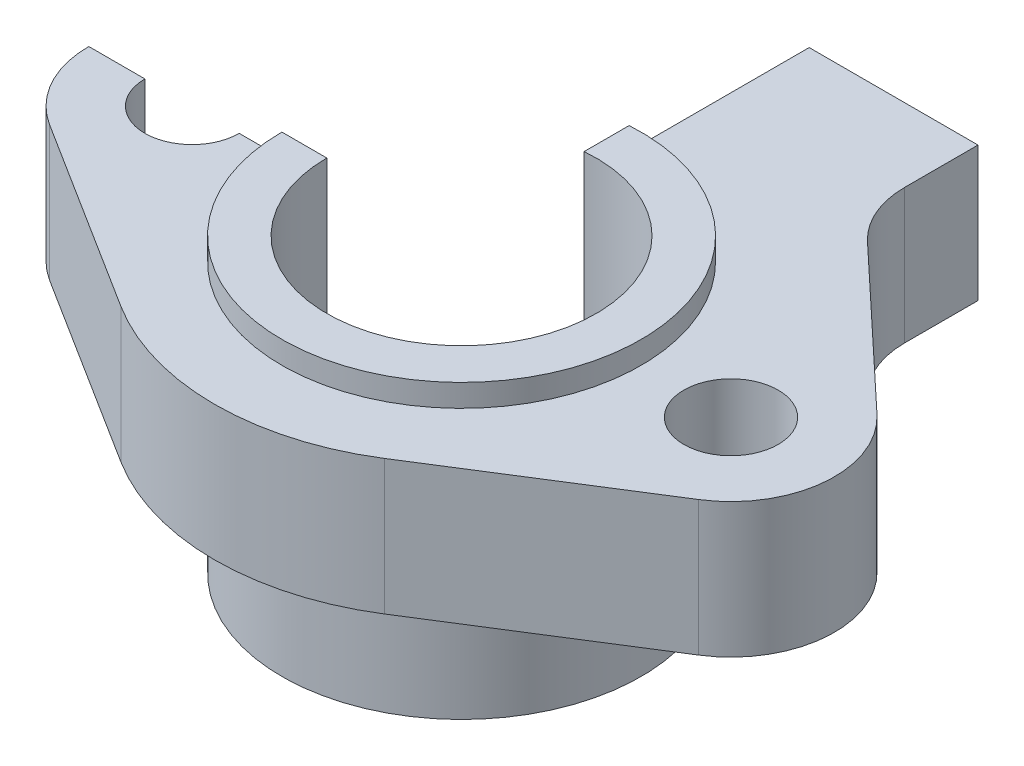
ISO-10303-21;
HEADER;
FILE_DESCRIPTION(('STEP AP214'),'2;1');
FILE_NAME('part.step','',(''),(''),'','','');
FILE_SCHEMA(('AUTOMOTIVE_DESIGN { 1 0 10303 214 1 1 1 1 }'));
ENDSEC;
DATA;
#1=APPLICATION_CONTEXT('core data for automotive mechanical design processes');
#2=APPLICATION_PROTOCOL_DEFINITION('international standard','automotive_design',2000,#1);
#3=PRODUCT_CONTEXT('',#1,'mechanical');
#4=PRODUCT('Part','Part','',(#3));
#5=PRODUCT_RELATED_PRODUCT_CATEGORY('part','',(#4));
#6=PRODUCT_DEFINITION_FORMATION('','',#4);
#7=PRODUCT_DEFINITION_CONTEXT('part definition',#1,'design');
#8=PRODUCT_DEFINITION('design','',#6,#7);
#9=PRODUCT_DEFINITION_SHAPE('','',#8);
#10=(LENGTH_UNIT() NAMED_UNIT(*) SI_UNIT(.MILLI.,.METRE.));
#11=(NAMED_UNIT(*) PLANE_ANGLE_UNIT() SI_UNIT($,.RADIAN.));
#12=(NAMED_UNIT(*) SI_UNIT($,.STERADIAN.) SOLID_ANGLE_UNIT());
#13=UNCERTAINTY_MEASURE_WITH_UNIT(LENGTH_MEASURE(1.E-05),#10,'distance_accuracy_value','');
#14=(GEOMETRIC_REPRESENTATION_CONTEXT(3) GLOBAL_UNCERTAINTY_ASSIGNED_CONTEXT((#13)) GLOBAL_UNIT_ASSIGNED_CONTEXT((#10,
#11,#12)) REPRESENTATION_CONTEXT('',''));
#15=CARTESIAN_POINT('',(0.,0.,0.));
#16=DIRECTION('',(0.,0.,1.));
#17=DIRECTION('',(1.,0.,0.));
#18=AXIS2_PLACEMENT_3D('',#15,#16,#17);
#19=CARTESIAN_POINT('',(0.,-135.,0.));
#20=DIRECTION('',(0.,0.,1.));
#21=DIRECTION('',(1.,0.,0.));
#22=AXIS2_PLACEMENT_3D('',#19,#20,#21);
#23=PLANE('',#22);
#24=DIRECTION('',(0.,1.,0.));
#25=VECTOR('',#24,1.);
#26=CARTESIAN_POINT('',(-49.5,-507.,0.));
#27=LINE('',#26,#25);
#28=CARTESIAN_POINT('',(-49.5,30.,0.));
#29=VERTEX_POINT('',#28);
#30=CARTESIAN_POINT('',(-49.5,0.,0.));
#31=VERTEX_POINT('',#30);
#32=EDGE_CURVE('E11',#29,#31,#27,.F.);
#33=ORIENTED_EDGE('',*,*,#32,.F.);
#34=DIRECTION('',(1.,0.,0.));
#35=VECTOR('',#34,1.);
#36=CARTESIAN_POINT('',(0.,30.,0.));
#37=LINE('',#36,#35);
#38=CARTESIAN_POINT('',(-40.,30.,0.));
#39=VERTEX_POINT('',#38);
#40=EDGE_CURVE('E63',#29,#39,#37,.T.);
#41=ORIENTED_EDGE('',*,*,#40,.T.);
#42=DIRECTION('',(0.,-1.,0.));
#43=VECTOR('',#42,1.);
#44=CARTESIAN_POINT('',(-40.,35.,0.));
#45=LINE('',#44,#43);
#46=CARTESIAN_POINT('',(-40.,35.,0.));
#47=VERTEX_POINT('',#46);
#48=EDGE_CURVE('E294',#47,#39,#45,.T.);
#49=ORIENTED_EDGE('',*,*,#48,.F.);
#50=DIRECTION('',(1.,0.,0.));
#51=VECTOR('',#50,1.);
#52=CARTESIAN_POINT('',(0.,35.,0.));
#53=LINE('',#52,#51);
#54=CARTESIAN_POINT('',(-30.,35.,0.));
#55=VERTEX_POINT('',#54);
#56=EDGE_CURVE('E302',#47,#55,#53,.T.);
#57=ORIENTED_EDGE('',*,*,#56,.T.);
#58=DIRECTION('',(0.,-1.,0.));
#59=VECTOR('',#58,1.);
#60=CARTESIAN_POINT('',(-30.,30.,0.));
#61=LINE('',#60,#59);
#62=CARTESIAN_POINT('',(-30.,-30.,0.));
#63=VERTEX_POINT('',#62);
#64=EDGE_CURVE('E308',#55,#63,#61,.T.);
#65=ORIENTED_EDGE('',*,*,#64,.T.);
#66=DIRECTION('',(1.,0.,0.));
#67=VECTOR('',#66,1.);
#68=CARTESIAN_POINT('',(0.,-30.,0.));
#69=LINE('',#68,#67);
#70=CARTESIAN_POINT('',(-40.,-30.,0.));
#71=VERTEX_POINT('',#70);
#72=EDGE_CURVE('E315',#71,#63,#69,.T.);
#73=ORIENTED_EDGE('',*,*,#72,.F.);
#74=DIRECTION('',(0.,-1.,0.));
#75=VECTOR('',#74,1.);
#76=CARTESIAN_POINT('',(-40.,30.,0.));
#77=LINE('',#76,#75);
#78=CARTESIAN_POINT('',(-40.,0.,0.));
#79=VERTEX_POINT('',#78);
#80=EDGE_CURVE('E190',#79,#71,#77,.T.);
#81=ORIENTED_EDGE('',*,*,#80,.F.);
#82=DIRECTION('',(1.,0.,0.));
#83=VECTOR('',#82,1.);
#84=CARTESIAN_POINT('',(0.,0.,0.));
#85=LINE('',#84,#83);
#86=EDGE_CURVE('E182',#31,#79,#85,.T.);
#87=ORIENTED_EDGE('',*,*,#86,.F.);
#88=EDGE_LOOP('',(#33,#41,#49,#57,#65,#73,#81,#87));
#89=FACE_BOUND('',#88,.T.);
#90=ADVANCED_FACE('F43',(#89),#23,.F.);
#91=DIRECTION('',(0.,1.,0.));
#92=VECTOR('',#91,1.);
#93=CARTESIAN_POINT('',(-70.5,-507.,0.));
#94=LINE('',#93,#92);
#95=CARTESIAN_POINT('',(-70.5,0.,0.));
#96=VERTEX_POINT('',#95);
#97=CARTESIAN_POINT('',(-70.5,30.,0.));
#98=VERTEX_POINT('',#97);
#99=EDGE_CURVE('E51',#96,#98,#94,.T.);
#100=ORIENTED_EDGE('',*,*,#99,.F.);
#101=CARTESIAN_POINT('',(-83.,0.,0.));
#102=VERTEX_POINT('',#101);
#103=EDGE_CURVE('E184',#102,#96,#85,.T.);
#104=ORIENTED_EDGE('',*,*,#103,.F.);
#105=DIRECTION('',(0.,1.,0.));
#106=VECTOR('',#105,1.);
#107=CARTESIAN_POINT('',(-83.,0.,0.));
#108=LINE('',#107,#106);
#109=CARTESIAN_POINT('',(-83.,30.,0.));
#110=VERTEX_POINT('',#109);
#111=EDGE_CURVE('E185',#102,#110,#108,.T.);
#112=ORIENTED_EDGE('',*,*,#111,.T.);
#113=EDGE_CURVE('E174',#110,#98,#37,.T.);
#114=ORIENTED_EDGE('',*,*,#113,.T.);
#115=EDGE_LOOP('',(#100,#104,#112,#114));
#116=FACE_BOUND('',#115,.T.);
#117=ADVANCED_FACE('F179',(#116),#23,.F.);
#118=CARTESIAN_POINT('',(0.,30.,0.));
#119=DIRECTION('',(0.,1.,0.));
#120=DIRECTION('',(0.,0.,1.));
#121=AXIS2_PLACEMENT_3D('',#118,#119,#120);
#122=PLANE('',#121);
#123=CARTESIAN_POINT('',(60.,30.,0.));
#124=DIRECTION('',(0.,1.,0.));
#125=DIRECTION('',(0.,0.,1.));
#126=AXIS2_PLACEMENT_3D('',#123,#124,#125);
#127=CIRCLE('',#126,10.5);
#128=CARTESIAN_POINT('',(60.,30.,10.5));
#129=VERTEX_POINT('',#128);
#130=EDGE_CURVE('E297',#129,#129,#127,.F.);
#131=ORIENTED_EDGE('',*,*,#130,.T.);
#132=EDGE_LOOP('',(#131));
#133=FACE_BOUND('',#132,.T.);
#134=ORIENTED_EDGE('',*,*,#40,.F.);
#135=CARTESIAN_POINT('',(-60.,30.,0.));
#136=DIRECTION('',(0.,1.,0.));
#137=DIRECTION('',(0.,0.,1.));
#138=AXIS2_PLACEMENT_3D('',#135,#136,#137);
#139=CIRCLE('',#138,10.5);
#140=EDGE_CURVE('E170',#29,#98,#139,.F.);
#141=ORIENTED_EDGE('',*,*,#140,.T.);
#142=ORIENTED_EDGE('',*,*,#113,.F.);
#143=CARTESIAN_POINT('',(-60.,30.,0.));
#144=DIRECTION('',(0.,1.,0.));
#145=DIRECTION('',(0.,0.,1.));
#146=AXIS2_PLACEMENT_3D('',#143,#144,#145);
#147=CIRCLE('',#146,23.);
#148=CARTESIAN_POINT('',(-72.2666666666667,30.,19.455818895356));
#149=VERTEX_POINT('',#148);
#150=EDGE_CURVE('E252',#110,#149,#147,.T.);
#151=ORIENTED_EDGE('',*,*,#150,.T.);
#152=DIRECTION('',(0.845905169363302,0.,0.533333333333333));
#153=VECTOR('',#152,1.);
#154=CARTESIAN_POINT('',(-29.3333333333333,30.,46.5247843149816));
#155=LINE('',#154,#153);
#156=CARTESIAN_POINT('',(-29.3333333333333,30.,46.5247843149816));
#157=VERTEX_POINT('',#156);
#158=EDGE_CURVE('E254',#149,#157,#155,.T.);
#159=ORIENTED_EDGE('',*,*,#158,.T.);
#160=CARTESIAN_POINT('',(0.,30.,0.));
#161=DIRECTION('',(0.,1.,0.));
#162=DIRECTION('',(0.,0.,1.));
#163=AXIS2_PLACEMENT_3D('',#160,#161,#162);
#164=CIRCLE('',#163,55.);
#165=CARTESIAN_POINT('',(29.3333333333333,30.,46.5247843149816));
#166=VERTEX_POINT('',#165);
#167=EDGE_CURVE('E257',#157,#166,#164,.T.);
#168=ORIENTED_EDGE('',*,*,#167,.T.);
#169=DIRECTION('',(0.845905169363301,0.,-0.533333333333334));
#170=VECTOR('',#169,1.);
#171=CARTESIAN_POINT('',(29.3333333333333,30.,46.5247843149816));
#172=LINE('',#171,#170);
#173=CARTESIAN_POINT('',(72.2666666666667,30.,19.4558188953559));
#174=VERTEX_POINT('',#173);
#175=EDGE_CURVE('E256',#166,#174,#172,.T.);
#176=ORIENTED_EDGE('',*,*,#175,.T.);
#177=CARTESIAN_POINT('',(60.,30.,0.));
#178=DIRECTION('',(0.,1.,0.));
#179=DIRECTION('',(0.,0.,1.));
#180=AXIS2_PLACEMENT_3D('',#177,#178,#179);
#181=CIRCLE('',#180,23.);
#182=CARTESIAN_POINT('',(75.7384595289657,30.,-16.7720270586208));
#183=VERTEX_POINT('',#182);
#184=EDGE_CURVE('E264',#174,#183,#181,.T.);
#185=ORIENTED_EDGE('',*,*,#184,.T.);
#186=DIRECTION('',(0.729218567766121,0.,0.684280849085466));
#187=VECTOR('',#186,1.);
#188=CARTESIAN_POINT('',(43.8328763544733,30.,-46.7114451018141));
#189=LINE('',#188,#187);
#190=CARTESIAN_POINT('',(41.3143830182907,30.,-49.0747375832144));
#191=VERTEX_POINT('',#190);
#192=EDGE_CURVE('E222',#191,#183,#189,.T.);
#193=ORIENTED_EDGE('',*,*,#192,.F.);
#194=CARTESIAN_POINT('',(55.,30.,-63.6591089385369));
#195=DIRECTION('',(0.,1.,0.));
#196=DIRECTION('',(0.,0.,1.));
#197=AXIS2_PLACEMENT_3D('',#194,#195,#196);
#198=CIRCLE('',#197,20.);
#199=CARTESIAN_POINT('',(35.,30.,-63.6591089385369));
#200=VERTEX_POINT('',#199);
#201=EDGE_CURVE('E219',#200,#191,#198,.T.);
#202=ORIENTED_EDGE('',*,*,#201,.F.);
#203=DIRECTION('',(0.,0.,1.));
#204=VECTOR('',#203,1.);
#205=CARTESIAN_POINT('',(35.,30.,0.));
#206=LINE('',#205,#204);
#207=CARTESIAN_POINT('',(35.,30.,-80.));
#208=VERTEX_POINT('',#207);
#209=EDGE_CURVE('E250',#208,#200,#206,.T.);
#210=ORIENTED_EDGE('',*,*,#209,.F.);
#211=DIRECTION('',(1.,0.,0.));
#212=VECTOR('',#211,1.);
#213=CARTESIAN_POINT('',(0.,30.,-80.));
#214=LINE('',#213,#212);
#215=CARTESIAN_POINT('',(-2.59305792163543,30.,-80.));
#216=VERTEX_POINT('',#215);
#217=EDGE_CURVE('E248',#216,#208,#214,.T.);
#218=ORIENTED_EDGE('',*,*,#217,.F.);
#219=DIRECTION('',(0.,0.,-1.));
#220=VECTOR('',#219,1.);
#221=CARTESIAN_POINT('',(-2.59305792163543,30.,0.));
#222=LINE('',#221,#220);
#223=CARTESIAN_POINT('',(-2.59305792163543,30.,-39.9158621429507));
#224=VERTEX_POINT('',#223);
#225=EDGE_CURVE('E205',#224,#216,#222,.T.);
#226=ORIENTED_EDGE('',*,*,#225,.F.);
#227=CARTESIAN_POINT('',(0.,30.,0.));
#228=DIRECTION('',(0.,1.,0.));
#229=DIRECTION('',(0.,0.,1.));
#230=AXIS2_PLACEMENT_3D('',#227,#228,#229);
#231=CIRCLE('',#230,40.);
#232=EDGE_CURVE('E214',#39,#224,#231,.T.);
#233=ORIENTED_EDGE('',*,*,#232,.F.);
#234=EDGE_LOOP('',(#134,#141,#142,#151,#159,#168,#176,#185,#193,#202,#210,#218,#226,#233));
#235=FACE_BOUND('',#234,.T.);
#236=ADVANCED_FACE('F172',(#133,#235),#122,.T.);
#237=CARTESIAN_POINT('',(0.,30.,0.));
#238=DIRECTION('',(0.,-1.,0.));
#239=DIRECTION('',(0.,0.,-1.));
#240=AXIS2_PLACEMENT_3D('',#237,#238,#239);
#241=CYLINDRICAL_SURFACE('',#240,40.);
#242=CARTESIAN_POINT('',(0.,-30.,0.));
#243=DIRECTION('',(0.,1.,0.));
#244=DIRECTION('',(0.,0.,1.));
#245=AXIS2_PLACEMENT_3D('',#242,#243,#244);
#246=CIRCLE('',#245,40.);
#247=CARTESIAN_POINT('',(-2.59305792163543,-30.,-39.9158621429507));
#248=VERTEX_POINT('',#247);
#249=EDGE_CURVE('E287',#71,#248,#246,.T.);
#250=ORIENTED_EDGE('',*,*,#249,.T.);
#251=DIRECTION('',(0.,-1.,0.));
#252=VECTOR('',#251,1.);
#253=CARTESIAN_POINT('',(-2.59305792163543,30.,-39.9158621429507));
#254=LINE('',#253,#252);
#255=CARTESIAN_POINT('',(-2.59305792163543,0.,-39.9158621429507));
#256=VERTEX_POINT('',#255);
#257=EDGE_CURVE('E200',#248,#256,#254,.F.);
#258=ORIENTED_EDGE('',*,*,#257,.T.);
#259=CARTESIAN_POINT('',(0.,0.,0.));
#260=DIRECTION('',(0.,1.,0.));
#261=DIRECTION('',(0.,0.,1.));
#262=AXIS2_PLACEMENT_3D('',#259,#260,#261);
#263=CIRCLE('',#262,40.);
#264=EDGE_CURVE('E292',#79,#256,#263,.T.);
#265=ORIENTED_EDGE('',*,*,#264,.F.);
#266=ORIENTED_EDGE('',*,*,#80,.T.);
#267=EDGE_LOOP('',(#250,#258,#265,#266));
#268=FACE_BOUND('',#267,.T.);
#269=ADVANCED_FACE('F44',(#268),#241,.T.);
#270=CARTESIAN_POINT('',(0.,-30.,0.));
#271=DIRECTION('',(0.,1.,0.));
#272=DIRECTION('',(0.,0.,1.));
#273=AXIS2_PLACEMENT_3D('',#270,#271,#272);
#274=PLANE('',#273);
#275=CARTESIAN_POINT('',(0.,-30.,0.));
#276=DIRECTION('',(0.,1.,0.));
#277=DIRECTION('',(0.,0.,1.));
#278=AXIS2_PLACEMENT_3D('',#275,#276,#277);
#279=CIRCLE('',#278,30.);
#280=CARTESIAN_POINT('',(-2.59305792163543,-30.,-29.8877240788763));
#281=VERTEX_POINT('',#280);
#282=EDGE_CURVE('E269',#63,#281,#279,.T.);
#283=ORIENTED_EDGE('',*,*,#282,.T.);
#284=DIRECTION('',(0.,0.,-1.));
#285=VECTOR('',#284,1.);
#286=CARTESIAN_POINT('',(-2.59305792163543,-30.,0.));
#287=LINE('',#286,#285);
#288=EDGE_CURVE('E198',#281,#248,#287,.T.);
#289=ORIENTED_EDGE('',*,*,#288,.T.);
#290=ORIENTED_EDGE('',*,*,#249,.F.);
#291=ORIENTED_EDGE('',*,*,#72,.T.);
#292=EDGE_LOOP('',(#283,#289,#290,#291));
#293=FACE_BOUND('',#292,.T.);
#294=ADVANCED_FACE('F325',(#293),#274,.F.);
#295=CARTESIAN_POINT('',(0.,30.,0.));
#296=DIRECTION('',(0.,-1.,0.));
#297=DIRECTION('',(0.,0.,-1.));
#298=AXIS2_PLACEMENT_3D('',#295,#296,#297);
#299=CYLINDRICAL_SURFACE('',#298,30.);
#300=DIRECTION('',(0.,-1.,0.));
#301=VECTOR('',#300,1.);
#302=CARTESIAN_POINT('',(-2.59305792163543,30.,-29.8877240788763));
#303=LINE('',#302,#301);
#304=CARTESIAN_POINT('',(-2.59305792163543,35.,-29.8877240788763));
#305=VERTEX_POINT('',#304);
#306=EDGE_CURVE('E191',#281,#305,#303,.F.);
#307=ORIENTED_EDGE('',*,*,#306,.F.);
#308=ORIENTED_EDGE('',*,*,#282,.F.);
#309=ORIENTED_EDGE('',*,*,#64,.F.);
#310=CARTESIAN_POINT('',(0.,35.,0.));
#311=DIRECTION('',(0.,1.,0.));
#312=DIRECTION('',(0.,0.,1.));
#313=AXIS2_PLACEMENT_3D('',#310,#311,#312);
#314=CIRCLE('',#313,30.);
#315=EDGE_CURVE('E208',#55,#305,#314,.T.);
#316=ORIENTED_EDGE('',*,*,#315,.T.);
#317=EDGE_LOOP('',(#307,#308,#309,#316));
#318=FACE_BOUND('',#317,.T.);
#319=ADVANCED_FACE('F327',(#318),#299,.F.);
#320=CARTESIAN_POINT('',(55.,0.,-63.6591089385369));
#321=DIRECTION('',(0.,1.,0.));
#322=DIRECTION('',(0.,0.,1.));
#323=AXIS2_PLACEMENT_3D('',#320,#321,#322);
#324=CYLINDRICAL_SURFACE('',#323,20.);
#325=ORIENTED_EDGE('',*,*,#201,.T.);
#326=DIRECTION('',(0.,1.,0.));
#327=VECTOR('',#326,1.);
#328=CARTESIAN_POINT('',(41.3143830182907,0.,-49.0747375832144));
#329=LINE('',#328,#327);
#330=CARTESIAN_POINT('',(41.3143830182907,0.,-49.0747375832144));
#331=VERTEX_POINT('',#330);
#332=EDGE_CURVE('E270',#331,#191,#329,.T.);
#333=ORIENTED_EDGE('',*,*,#332,.F.);
#334=CARTESIAN_POINT('',(55.,0.,-63.6591089385369));
#335=DIRECTION('',(0.,1.,0.));
#336=DIRECTION('',(0.,0.,1.));
#337=AXIS2_PLACEMENT_3D('',#334,#335,#336);
#338=CIRCLE('',#337,20.);
#339=CARTESIAN_POINT('',(35.,0.,-63.6591089385369));
#340=VERTEX_POINT('',#339);
#341=EDGE_CURVE('E216',#340,#331,#338,.T.);
#342=ORIENTED_EDGE('',*,*,#341,.F.);
#343=DIRECTION('',(0.,1.,0.));
#344=VECTOR('',#343,1.);
#345=CARTESIAN_POINT('',(35.,0.,-63.6591089385369));
#346=LINE('',#345,#344);
#347=EDGE_CURVE('E242',#340,#200,#346,.T.);
#348=ORIENTED_EDGE('',*,*,#347,.T.);
#349=EDGE_LOOP('',(#325,#333,#342,#348));
#350=FACE_BOUND('',#349,.T.);
#351=ADVANCED_FACE('F375',(#350),#324,.F.);
#352=CARTESIAN_POINT('',(43.8328763544733,0.,-46.7114451018141));
#353=DIRECTION('',(-0.684280849085466,0.,0.729218567766121));
#354=DIRECTION('',(0.729218567766121,0.,0.684280849085466));
#355=AXIS2_PLACEMENT_3D('',#352,#353,#354);
#356=PLANE('',#355);
#357=ORIENTED_EDGE('',*,*,#192,.T.);
#358=DIRECTION('',(0.,1.,0.));
#359=VECTOR('',#358,1.);
#360=CARTESIAN_POINT('',(75.7384595289657,0.,-16.7720270586208));
#361=LINE('',#360,#359);
#362=CARTESIAN_POINT('',(75.7384595289657,0.,-16.7720270586208));
#363=VERTEX_POINT('',#362);
#364=EDGE_CURVE('E272',#363,#183,#361,.T.);
#365=ORIENTED_EDGE('',*,*,#364,.F.);
#366=DIRECTION('',(0.729218567766121,0.,0.684280849085466));
#367=VECTOR('',#366,1.);
#368=CARTESIAN_POINT('',(43.8328763544733,0.,-46.7114451018141));
#369=LINE('',#368,#367);
#370=EDGE_CURVE('E245',#331,#363,#369,.T.);
#371=ORIENTED_EDGE('',*,*,#370,.F.);
#372=ORIENTED_EDGE('',*,*,#332,.T.);
#373=EDGE_LOOP('',(#357,#365,#371,#372));
#374=FACE_BOUND('',#373,.T.);
#375=ADVANCED_FACE('F368',(#374),#356,.F.);
#376=CARTESIAN_POINT('',(60.,0.,0.));
#377=DIRECTION('',(0.,1.,0.));
#378=DIRECTION('',(0.,0.,1.));
#379=AXIS2_PLACEMENT_3D('',#376,#377,#378);
#380=CYLINDRICAL_SURFACE('',#379,23.);
#381=ORIENTED_EDGE('',*,*,#184,.F.);
#382=DIRECTION('',(0.,1.,0.));
#383=VECTOR('',#382,1.);
#384=CARTESIAN_POINT('',(72.2666666666667,0.,19.4558188953559));
#385=LINE('',#384,#383);
#386=CARTESIAN_POINT('',(72.2666666666667,0.,19.4558188953559));
#387=VERTEX_POINT('',#386);
#388=EDGE_CURVE('E271',#387,#174,#385,.T.);
#389=ORIENTED_EDGE('',*,*,#388,.F.);
#390=CARTESIAN_POINT('',(60.,0.,0.));
#391=DIRECTION('',(0.,1.,0.));
#392=DIRECTION('',(0.,0.,1.));
#393=AXIS2_PLACEMENT_3D('',#390,#391,#392);
#394=CIRCLE('',#393,23.);
#395=EDGE_CURVE('E237',#387,#363,#394,.T.);
#396=ORIENTED_EDGE('',*,*,#395,.T.);
#397=ORIENTED_EDGE('',*,*,#364,.T.);
#398=EDGE_LOOP('',(#381,#389,#396,#397));
#399=FACE_BOUND('',#398,.T.);
#400=ADVANCED_FACE('F371',(#399),#380,.T.);
#401=CARTESIAN_POINT('',(29.3333333333333,0.,46.5247843149816));
#402=DIRECTION('',(0.533333333333334,0.,0.845905169363301));
#403=DIRECTION('',(0.845905169363301,0.,-0.533333333333334));
#404=AXIS2_PLACEMENT_3D('',#401,#402,#403);
#405=PLANE('',#404);
#406=ORIENTED_EDGE('',*,*,#175,.F.);
#407=DIRECTION('',(0.,1.,0.));
#408=VECTOR('',#407,1.);
#409=CARTESIAN_POINT('',(29.3333333333333,0.,46.5247843149816));
#410=LINE('',#409,#408);
#411=CARTESIAN_POINT('',(29.3333333333333,0.,46.5247843149816));
#412=VERTEX_POINT('',#411);
#413=EDGE_CURVE('E273',#412,#166,#410,.T.);
#414=ORIENTED_EDGE('',*,*,#413,.F.);
#415=DIRECTION('',(0.845905169363301,0.,-0.533333333333334));
#416=VECTOR('',#415,1.);
#417=CARTESIAN_POINT('',(29.3333333333333,0.,46.5247843149816));
#418=LINE('',#417,#416);
#419=EDGE_CURVE('E236',#412,#387,#418,.T.);
#420=ORIENTED_EDGE('',*,*,#419,.T.);
#421=ORIENTED_EDGE('',*,*,#388,.T.);
#422=EDGE_LOOP('',(#406,#414,#420,#421));
#423=FACE_BOUND('',#422,.T.);
#424=ADVANCED_FACE('F376',(#423),#405,.T.);
#425=CARTESIAN_POINT('',(0.,0.,0.));
#426=DIRECTION('',(0.,1.,0.));
#427=DIRECTION('',(0.,0.,1.));
#428=AXIS2_PLACEMENT_3D('',#425,#426,#427);
#429=CYLINDRICAL_SURFACE('',#428,55.);
#430=ORIENTED_EDGE('',*,*,#167,.F.);
#431=DIRECTION('',(0.,1.,0.));
#432=VECTOR('',#431,1.);
#433=CARTESIAN_POINT('',(-29.3333333333333,0.,46.5247843149816));
#434=LINE('',#433,#432);
#435=CARTESIAN_POINT('',(-29.3333333333333,0.,46.5247843149816));
#436=VERTEX_POINT('',#435);
#437=EDGE_CURVE('E280',#436,#157,#434,.T.);
#438=ORIENTED_EDGE('',*,*,#437,.F.);
#439=CARTESIAN_POINT('',(0.,0.,0.));
#440=DIRECTION('',(0.,1.,0.));
#441=DIRECTION('',(0.,0.,1.));
#442=AXIS2_PLACEMENT_3D('',#439,#440,#441);
#443=CIRCLE('',#442,55.);
#444=EDGE_CURVE('E231',#436,#412,#443,.T.);
#445=ORIENTED_EDGE('',*,*,#444,.T.);
#446=ORIENTED_EDGE('',*,*,#413,.T.);
#447=EDGE_LOOP('',(#430,#438,#445,#446));
#448=FACE_BOUND('',#447,.T.);
#449=ADVANCED_FACE('F379',(#448),#429,.T.);
#450=CARTESIAN_POINT('',(-29.3333333333333,0.,46.5247843149816));
#451=DIRECTION('',(-0.533333333333333,0.,0.845905169363301));
#452=DIRECTION('',(0.845905169363301,0.,0.533333333333333));
#453=AXIS2_PLACEMENT_3D('',#450,#451,#452);
#454=PLANE('',#453);
#455=ORIENTED_EDGE('',*,*,#158,.F.);
#456=DIRECTION('',(0.,1.,0.));
#457=VECTOR('',#456,1.);
#458=CARTESIAN_POINT('',(-72.2666666666667,0.,19.455818895356));
#459=LINE('',#458,#457);
#460=CARTESIAN_POINT('',(-72.2666666666667,0.,19.455818895356));
#461=VERTEX_POINT('',#460);
#462=EDGE_CURVE('E276',#461,#149,#459,.T.);
#463=ORIENTED_EDGE('',*,*,#462,.F.);
#464=DIRECTION('',(0.845905169363302,0.,0.533333333333333));
#465=VECTOR('',#464,1.);
#466=CARTESIAN_POINT('',(-29.3333333333333,0.,46.5247843149816));
#467=LINE('',#466,#465);
#468=EDGE_CURVE('E229',#461,#436,#467,.T.);
#469=ORIENTED_EDGE('',*,*,#468,.T.);
#470=ORIENTED_EDGE('',*,*,#437,.T.);
#471=EDGE_LOOP('',(#455,#463,#469,#470));
#472=FACE_BOUND('',#471,.T.);
#473=ADVANCED_FACE('F381',(#472),#454,.T.);
#474=CARTESIAN_POINT('',(-60.,0.,0.));
#475=DIRECTION('',(0.,1.,0.));
#476=DIRECTION('',(0.,0.,1.));
#477=AXIS2_PLACEMENT_3D('',#474,#475,#476);
#478=CYLINDRICAL_SURFACE('',#477,23.);
#479=ORIENTED_EDGE('',*,*,#111,.F.);
#480=CARTESIAN_POINT('',(-60.,0.,0.));
#481=DIRECTION('',(0.,1.,0.));
#482=DIRECTION('',(0.,0.,1.));
#483=AXIS2_PLACEMENT_3D('',#480,#481,#482);
#484=CIRCLE('',#483,23.);
#485=EDGE_CURVE('E226',#102,#461,#484,.T.);
#486=ORIENTED_EDGE('',*,*,#485,.T.);
#487=ORIENTED_EDGE('',*,*,#462,.T.);
#488=ORIENTED_EDGE('',*,*,#150,.F.);
#489=EDGE_LOOP('',(#479,#486,#487,#488));
#490=FACE_BOUND('',#489,.T.);
#491=ADVANCED_FACE('F389',(#490),#478,.T.);
#492=CARTESIAN_POINT('',(0.,0.,-80.));
#493=DIRECTION('',(0.,0.,1.));
#494=DIRECTION('',(1.,0.,0.));
#495=AXIS2_PLACEMENT_3D('',#492,#493,#494);
#496=PLANE('',#495);
#497=DIRECTION('',(1.,0.,0.));
#498=VECTOR('',#497,1.);
#499=CARTESIAN_POINT('',(0.,0.,-80.));
#500=LINE('',#499,#498);
#501=CARTESIAN_POINT('',(-2.59305792163543,0.,-80.));
#502=VERTEX_POINT('',#501);
#503=CARTESIAN_POINT('',(35.,0.,-80.));
#504=VERTEX_POINT('',#503);
#505=EDGE_CURVE('E228',#502,#504,#500,.T.);
#506=ORIENTED_EDGE('',*,*,#505,.F.);
#507=DIRECTION('',(0.,1.,0.));
#508=VECTOR('',#507,1.);
#509=CARTESIAN_POINT('',(-2.59305792163543,0.,-80.));
#510=LINE('',#509,#508);
#511=EDGE_CURVE('E210',#502,#216,#510,.T.);
#512=ORIENTED_EDGE('',*,*,#511,.T.);
#513=ORIENTED_EDGE('',*,*,#217,.T.);
#514=DIRECTION('',(0.,1.,0.));
#515=VECTOR('',#514,1.);
#516=CARTESIAN_POINT('',(35.,0.,-80.));
#517=LINE('',#516,#515);
#518=EDGE_CURVE('E284',#504,#208,#517,.T.);
#519=ORIENTED_EDGE('',*,*,#518,.F.);
#520=EDGE_LOOP('',(#506,#512,#513,#519));
#521=FACE_BOUND('',#520,.T.);
#522=ADVANCED_FACE('F345',(#521),#496,.F.);
#523=CARTESIAN_POINT('',(35.,0.,0.));
#524=DIRECTION('',(-1.,0.,0.));
#525=DIRECTION('',(0.,0.,1.));
#526=AXIS2_PLACEMENT_3D('',#523,#524,#525);
#527=PLANE('',#526);
#528=ORIENTED_EDGE('',*,*,#209,.T.);
#529=ORIENTED_EDGE('',*,*,#347,.F.);
#530=DIRECTION('',(0.,0.,1.));
#531=VECTOR('',#530,1.);
#532=CARTESIAN_POINT('',(35.,0.,0.));
#533=LINE('',#532,#531);
#534=EDGE_CURVE('E221',#504,#340,#533,.T.);
#535=ORIENTED_EDGE('',*,*,#534,.F.);
#536=ORIENTED_EDGE('',*,*,#518,.T.);
#537=EDGE_LOOP('',(#528,#529,#535,#536));
#538=FACE_BOUND('',#537,.T.);
#539=ADVANCED_FACE('F370',(#538),#527,.F.);
#540=CARTESIAN_POINT('',(0.,0.,0.));
#541=DIRECTION('',(0.,1.,0.));
#542=DIRECTION('',(0.,0.,1.));
#543=AXIS2_PLACEMENT_3D('',#540,#541,#542);
#544=PLANE('',#543);
#545=CARTESIAN_POINT('',(-60.,0.,0.));
#546=DIRECTION('',(0.,1.,0.));
#547=DIRECTION('',(0.,0.,1.));
#548=AXIS2_PLACEMENT_3D('',#545,#546,#547);
#549=CIRCLE('',#548,10.5);
#550=EDGE_CURVE('E60',#31,#96,#549,.F.);
#551=ORIENTED_EDGE('',*,*,#550,.F.);
#552=ORIENTED_EDGE('',*,*,#86,.T.);
#553=ORIENTED_EDGE('',*,*,#264,.T.);
#554=DIRECTION('',(0.,0.,-1.));
#555=VECTOR('',#554,1.);
#556=CARTESIAN_POINT('',(-2.59305792163543,0.,0.));
#557=LINE('',#556,#555);
#558=EDGE_CURVE('E202',#256,#502,#557,.T.);
#559=ORIENTED_EDGE('',*,*,#558,.T.);
#560=ORIENTED_EDGE('',*,*,#505,.T.);
#561=ORIENTED_EDGE('',*,*,#534,.T.);
#562=ORIENTED_EDGE('',*,*,#341,.T.);
#563=ORIENTED_EDGE('',*,*,#370,.T.);
#564=ORIENTED_EDGE('',*,*,#395,.F.);
#565=ORIENTED_EDGE('',*,*,#419,.F.);
#566=ORIENTED_EDGE('',*,*,#444,.F.);
#567=ORIENTED_EDGE('',*,*,#468,.F.);
#568=ORIENTED_EDGE('',*,*,#485,.F.);
#569=ORIENTED_EDGE('',*,*,#103,.T.);
#570=EDGE_LOOP('',(#551,#552,#553,#559,#560,#561,#562,#563,#564,#565,#566,#567,#568,#569));
#571=FACE_BOUND('',#570,.T.);
#572=CARTESIAN_POINT('',(60.,0.,0.));
#573=DIRECTION('',(0.,1.,0.));
#574=DIRECTION('',(0.,0.,1.));
#575=AXIS2_PLACEMENT_3D('',#572,#573,#574);
#576=CIRCLE('',#575,10.5);
#577=CARTESIAN_POINT('',(60.,0.,10.5));
#578=VERTEX_POINT('',#577);
#579=EDGE_CURVE('E178',#578,#578,#576,.F.);
#580=ORIENTED_EDGE('',*,*,#579,.F.);
#581=EDGE_LOOP('',(#580));
#582=FACE_BOUND('',#581,.T.);
#583=ADVANCED_FACE('F348',(#571,#582),#544,.F.);
#584=CARTESIAN_POINT('',(0.,35.,0.));
#585=DIRECTION('',(0.,1.,0.));
#586=DIRECTION('',(0.,0.,1.));
#587=AXIS2_PLACEMENT_3D('',#584,#585,#586);
#588=PLANE('',#587);
#589=DIRECTION('',(0.,0.,-1.));
#590=VECTOR('',#589,1.);
#591=CARTESIAN_POINT('',(-2.59305792163543,35.,0.));
#592=LINE('',#591,#590);
#593=CARTESIAN_POINT('',(-2.59305792163543,35.,-39.9158621429507));
#594=VERTEX_POINT('',#593);
#595=EDGE_CURVE('E195',#305,#594,#592,.T.);
#596=ORIENTED_EDGE('',*,*,#595,.F.);
#597=ORIENTED_EDGE('',*,*,#315,.F.);
#598=ORIENTED_EDGE('',*,*,#56,.F.);
#599=CARTESIAN_POINT('',(0.,35.,0.));
#600=DIRECTION('',(0.,1.,0.));
#601=DIRECTION('',(0.,0.,1.));
#602=AXIS2_PLACEMENT_3D('',#599,#600,#601);
#603=CIRCLE('',#602,40.);
#604=EDGE_CURVE('E211',#47,#594,#603,.T.);
#605=ORIENTED_EDGE('',*,*,#604,.T.);
#606=EDGE_LOOP('',(#596,#597,#598,#605));
#607=FACE_BOUND('',#606,.T.);
#608=ADVANCED_FACE('F331',(#607),#588,.T.);
#609=CARTESIAN_POINT('',(0.,35.,0.));
#610=DIRECTION('',(0.,-1.,0.));
#611=DIRECTION('',(0.,0.,-1.));
#612=AXIS2_PLACEMENT_3D('',#609,#610,#611);
#613=CYLINDRICAL_SURFACE('',#612,40.);
#614=ORIENTED_EDGE('',*,*,#232,.T.);
#615=DIRECTION('',(0.,-1.,0.));
#616=VECTOR('',#615,1.);
#617=CARTESIAN_POINT('',(-2.59305792163543,35.,-39.9158621429507));
#618=LINE('',#617,#616);
#619=EDGE_CURVE('E171',#224,#594,#618,.F.);
#620=ORIENTED_EDGE('',*,*,#619,.T.);
#621=ORIENTED_EDGE('',*,*,#604,.F.);
#622=ORIENTED_EDGE('',*,*,#48,.T.);
#623=EDGE_LOOP('',(#614,#620,#621,#622));
#624=FACE_BOUND('',#623,.T.);
#625=ADVANCED_FACE('F340',(#624),#613,.T.);
#626=CARTESIAN_POINT('',(-2.59305792163543,-135.,0.));
#627=DIRECTION('',(1.,0.,0.));
#628=DIRECTION('',(0.,0.,-1.));
#629=AXIS2_PLACEMENT_3D('',#626,#627,#628);
#630=PLANE('',#629);
#631=ORIENTED_EDGE('',*,*,#558,.F.);
#632=ORIENTED_EDGE('',*,*,#257,.F.);
#633=ORIENTED_EDGE('',*,*,#288,.F.);
#634=ORIENTED_EDGE('',*,*,#306,.T.);
#635=ORIENTED_EDGE('',*,*,#595,.T.);
#636=ORIENTED_EDGE('',*,*,#619,.F.);
#637=ORIENTED_EDGE('',*,*,#225,.T.);
#638=ORIENTED_EDGE('',*,*,#511,.F.);
#639=EDGE_LOOP('',(#631,#632,#633,#634,#635,#636,#637,#638));
#640=FACE_BOUND('',#639,.T.);
#641=ADVANCED_FACE('F323',(#640),#630,.F.);
#642=CARTESIAN_POINT('',(60.,-99.,0.));
#643=DIRECTION('',(0.,1.,0.));
#644=DIRECTION('',(0.,0.,1.));
#645=AXIS2_PLACEMENT_3D('',#642,#643,#644);
#646=CYLINDRICAL_SURFACE('',#645,10.5);
#647=ORIENTED_EDGE('',*,*,#130,.F.);
#648=EDGE_LOOP('',(#647));
#649=FACE_BOUND('',#648,.T.);
#650=ORIENTED_EDGE('',*,*,#579,.T.);
#651=EDGE_LOOP('',(#650));
#652=FACE_BOUND('',#651,.T.);
#653=ADVANCED_FACE('F357',(#649,#652),#646,.F.);
#654=CARTESIAN_POINT('',(-60.,-507.,0.));
#655=DIRECTION('',(0.,1.,0.));
#656=DIRECTION('',(0.,0.,1.));
#657=AXIS2_PLACEMENT_3D('',#654,#655,#656);
#658=CYLINDRICAL_SURFACE('',#657,10.5);
#659=ORIENTED_EDGE('',*,*,#32,.T.);
#660=ORIENTED_EDGE('',*,*,#550,.T.);
#661=ORIENTED_EDGE('',*,*,#99,.T.);
#662=ORIENTED_EDGE('',*,*,#140,.F.);
#663=EDGE_LOOP('',(#659,#660,#661,#662));
#664=FACE_BOUND('',#663,.T.);
#665=ADVANCED_FACE('F168',(#664),#658,.F.);
#666=CLOSED_SHELL('',(#90,#117,#236,#269,#294,#319,#351,#375,#400,#424,#449,#473,#491,#522,#539,
#583,#608,#625,#641,#653,#665));
#667=MANIFOLD_SOLID_BREP('B2',#666);
#668=ADVANCED_BREP_SHAPE_REPRESENTATION('',(#18,#667),#14);
#669=SHAPE_DEFINITION_REPRESENTATION(#9,#668);
ENDSEC;
END-ISO-10303-21;
